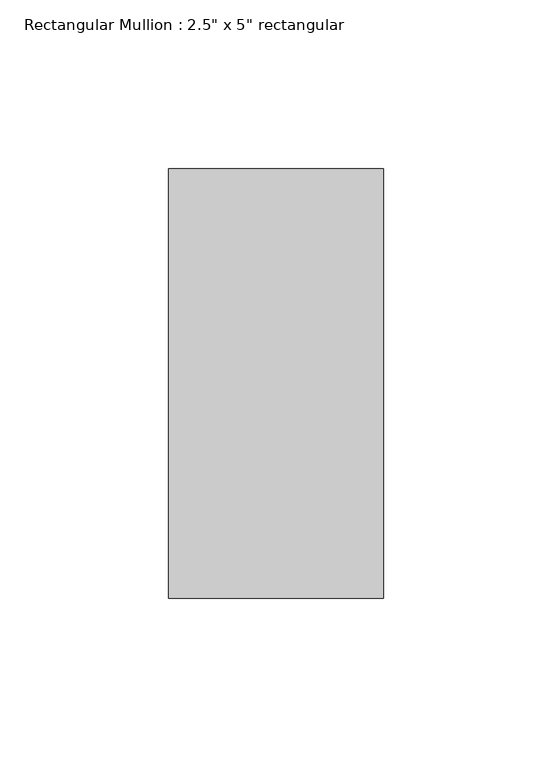
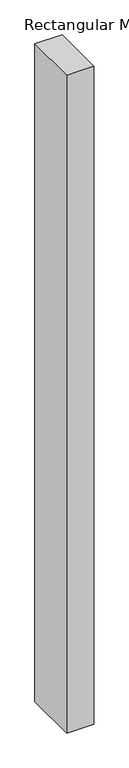
"""IFC4 building model written with IfcOpenShell, lengths in millimetres: member geometry."""

from ifc_helpers import new_model, si_unit, frame, origin, place, context, project, spatial, polyline, outline, extrude, source, transform, mapped, element, save


def member_780c4c5d(model_context):
    return source(origin(), model_context, "Body", "SweptSolid", [
        extrude(outline(polyline([(31.75, 63.5), (31.75, -63.5), (-31.75, -63.5), (-31.75, 63.5), (31.75, 63.5)])), frame((0.0, 0.0, -1611.1494203), z_axis=(0.0, 0.0, 1.0), x_axis=(1.0, 0.0, 0.0)), (0.0, 0.0, 1.0), 1611.1494203),
    ])


if __name__ == "__main__":
    model = new_model("IFC4")
    model_context = context("Model", 3, world=origin())
    ifc_project = project(units=[si_unit("LENGTHUNIT", "METRE", prefix="MILLI")], contexts=[model_context])
    site = spatial("IfcSite", under=ifc_project)
    building = spatial("IfcBuilding", under=site)
    placement = place(None, origin())
    member_shape = member_780c4c5d(model_context)
    element("IfcMember", 1, ObjectType="Rectangular Mullion : 2.5\" x 5\" rectangular", at=placement, inside=building, context=model_context, shape_type="MappedRepresentation", body=[
        mapped(member_shape, transform((0.0, 0.0, 0.0), x_axis=(1.0, 0.0, 0.0), y_axis=(0.0, 1.0, 0.0), z_axis=(0.0, 0.0, 1.0))),
    ])
    save(model, "model.ifc")

# Revit data of these elements
# Type "Rectangular Mullion : 2.5\" x 5\" rectangular"
#   built-in parameter 1007304 = 0.416667 (stored number, unit not read)
#   built-in parameter 1007301 = 0.104167 (stored number, unit not read)
#   built-in parameter 1007300 = 0.104167 (stored number, unit not read)
# Element 1 (IfcMember, "Rectangular Mullion : 2.5\" x 5\" rectangular")
#   Materials on its faces: "Aluminum"
# Materials
#   "Aluminum": class "Metal", colour RGB 247 247 247, transparency 0, Description = "Aluminum 6061", Cost = 0
